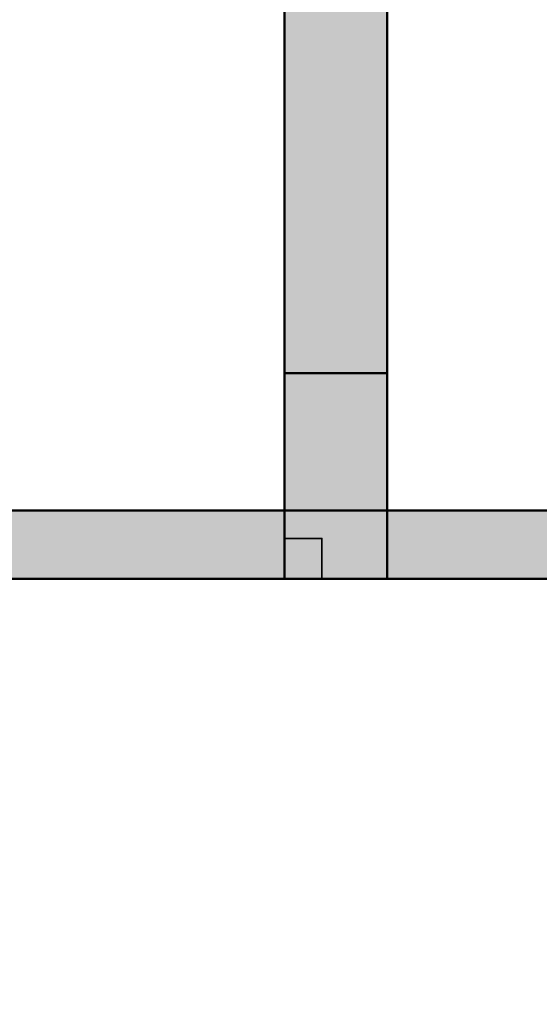
# Model space of a CAD drawing. Units: inches. Extents: x -7 to 1228, y -146 to 1091.
# Tile 64 of 88: x 611 to 656, y 531 to 617. Entities that reach past the tile are written whole.
import ezdxf

# ---------------------------------------------------------------- set-up
doc = ezdxf.new("R2010")
doc.units = ezdxf.units.IN
for name, color, linetype, lineweight in [('A-COLS', 6, 'Continuous', 35), ('A-WALL', 7, 'Continuous', 50), ('A-WALL-PATT', 251, 'Continuous', 13)]:
    doc.layers.add(name, color=color, linetype=linetype, lineweight=lineweight)

msp = doc.modelspace()

# ---------------------------------------------------------------- hatches: boundary and pattern name
at = {"layer": 'A-COLS'}
h = msp.add_hatch(color=256, dxfattribs=at)
h.dxf.hatch_style = 1
h.paths.add_polyline_path([(643, 586), (634, 586), (634, 571.546), (637.289, 571.546), (637.289, 568), (643, 568)])
h = msp.add_hatch(color=256, dxfattribs=at)
h.dxf.hatch_style = 1
h.paths.add_polyline_path([(637.289, 571.546), (634, 571.546), (634, 568), (637.289, 568)])
at = {"layer": 'A-WALL-PATT'}
h = msp.add_hatch(color=256, dxfattribs=at)
h.dxf.hatch_style = 1
h.paths.add_polyline_path([(69, 568), (60, 568), (60, 493), (63.289, 493), (69, 493)])
h.paths.add_polyline_path([(69, 662.405), (60, 662.405), (60, 586), (69, 586)], flags=17)
h.paths.add_polyline_path([(69, 723), (184, 723), (184, 734), (179, 734), (179, 728), (69, 728), (69, 741.623), (60, 741.623), (60, 698.405), (69, 698.405)], flags=17)
h.paths.add_polyline_path([(69, 782), (231, 782), (231, 728), (231, 723), (231, 586), (236, 586), (236, 787), (69, 787), (69, 800.126), (60, 800.126), (60, 765.623), (69, 765.623)])
h.paths.add_polyline_path([(184, 842), (189, 842), (189, 848), (173, 848), (173, 842), (179, 842), (179, 787), (184, 787)])
h.paths.add_polyline_path([(118.22, 69), (69, 69), (69, 60), (118.22, 60)])
h.paths.add_polyline_path([(227, 69), (154.22, 69), (154.22, 60), (227, 60)])
h.paths.add_polyline_path([(236, 60), (232.711, 60), (227, 60), (227, 36), (236, 36)])
h.paths.add_polyline_path([(389, 60), (380, 60), (380, 36), (389, 36)])
h.paths.add_polyline_path([(384, 181), (380, 181), (380, 115), (380, 78), (384, 78)])
h.paths.add_polyline_path([(380, 115), (334.547, 115), (334.547, 109), (380, 109)])
h.paths.add_polyline_path([(274.547, 115), (236, 115), (236, 201), (232.711, 201), (231, 201), (231, 78), (236, 78), (236, 109), (274.547, 109)])
h.paths.add_polyline_path([(69, 123), (60, 123), (60, 78), (69, 78)])
h.paths.add_polyline_path([(69, 201), (60, 201), (60, 159), (69, 159)])
h.paths.add_polyline_path([(143, 219), (69, 219), (69, 213), (143, 213)], flags=17)
h.paths.add_polyline_path([(189, 219), (184, 219), (184, 274), (231, 274), (231, 219), (236, 219), (236, 279), (184, 279), (184, 297), (179, 297), (179, 279), (69, 279), (69, 290.912), (60, 290.912), (60, 262.179), (69, 262.179), (69, 274), (179, 274), (179, 219), (173, 219), (173, 213), (189, 213)])
h.paths.add_polyline_path([(69, 238.179), (60, 238.179), (60, 219), (69, 219)], flags=17)
h.paths.add_polyline_path([(69, 333), (60, 333), (60, 314.912), (69, 314.912), (69, 316.965)])
h.paths.add_polyline_path([(190, 338), (184, 338), (69, 338), (69, 333), (179, 333), (179, 327), (184, 327), (184, 333.021), (190, 333.046)])
h.paths.add_polyline_path([(69, 386.806), (60, 386.806), (60, 351), (69, 351)])
h.paths.add_polyline_path([(69, 475), (60, 475), (60, 422.806), (69, 422.806)])
h.paths.add_polyline_path([(236, 475), (231, 475), (231, 351.238), (236, 351.238)])
h.paths.add_polyline_path([(384, 475), (380, 475), (380, 362), (384, 362)])
h.paths.add_polyline_path([(547, 307), (439, 307), (439, 356), (445, 356), (445, 362), (433, 362), (433, 307), (380, 307), (380, 244), (380, 241), (384, 241), (384, 301), (433, 301), (433, 277), (439, 277), (439, 301), (547, 301)])
h.paths.add_polyline_path([(547, 241), (439, 241), (439, 247), (433, 247), (433, 235), (547, 235)])
h.paths.add_polyline_path([(450, 69), (440.286, 69), (424.889, 69), (389, 69), (389, 60), (450, 60)])
h.paths.add_polyline_path([(547, 69), (486, 69), (486, 60), (547, 60)])
h.paths.add_polyline_path([(556, 148.268), (547, 148.268), (547, 78), (556, 78)])
h.paths.add_polyline_path([(556, 223), (547, 223), (547, 195), (547, 184.268), (556, 184.268)])
h.paths.add_polyline_path([(556, 311.192), (547, 311.192), (547, 273.075), (556, 273.075)])
h.paths.add_polyline_path([(556, 344), (552.711, 344), (547, 344), (547, 335.192), (556, 335.192)])
h.paths.add_polyline_path([(556, 249.075), (547, 249.075), (547, 241), (556, 241)])
h.paths.add_polyline_path([(547, 362), (475, 362), (475, 356), (547, 356)], flags=0)
h.paths.add_polyline_path([(556, 399.621), (547, 399.621), (547, 362), (556, 362)])
h.paths.add_polyline_path([(556, 475), (547, 475), (547, 435.621), (556, 435.621)])
h.paths.add_polyline_path([(547, 493), (389, 493), (389, 487), (547, 487)])
h.paths.add_polyline_path([(380, 493), (278, 493), (278, 487), (380, 487)])
h.paths.add_polyline_path([(227, 493), (69, 493), (69, 487), (227, 487)])
h.paths.add_polyline_path([(643, 122.445), (634, 122.445), (634, 78), (643, 78)])
h.paths.add_polyline_path([(702.5, 69), (692.786, 69), (677.389, 69), (643, 69), (643, 60), (702.5, 60)])
h.paths.add_polyline_path([(798, 69), (738.5, 69), (738.5, 60), (798, 60)])
h.paths.add_polyline_path([(807, 60), (803.711, 60), (798, 60), (798, 36), (807, 36)])
h.paths.add_polyline_path([(807, 109), (846.751, 109), (846.751, 115), (807, 115), (807, 159), (802, 159), (802, 78), (807, 78)])
h.paths.add_polyline_path([(807, 201), (802, 201), (802, 195), (807, 195)])
h.paths.add_polyline_path([(643, 201), (634, 201), (634, 158.445), (643, 158.445)])
h.paths.add_polyline_path([(756, 225), (751, 225), (751, 219), (643, 219), (643, 213), (756, 213)])
h.paths.add_polyline_path([(643, 240.848), (634, 240.848), (634, 219), (643, 219)])
h.paths.add_polyline_path([(643, 274), (643, 288.629), (634, 288.629), (634, 264.848), (643, 264.848)])
h.paths.add_polyline_path([(802, 279), (756, 279), (756, 297), (751, 297), (751, 279), (643, 279), (643, 274), (751, 274), (751, 255), (756, 255), (756, 274), (802, 274)])
h.paths.add_polyline_path([(807, 333), (803.711, 333), (802, 333), (802, 279), (802, 274), (802, 219), (807, 219)])
h.paths.add_polyline_path([(956, 182), (951, 182), (951, 115), (906.751, 115), (906.751, 109), (951, 109), (951, 78), (956, 78)])
h.paths.add_polyline_path([(960, 60), (951, 60), (951, 36), (960, 36)])
h.paths.add_polyline_path([(1021, 69), (1005.781, 69), (960, 69), (960, 60), (1021, 60)])
h.paths.add_polyline_path([(956, 224), (951, 224), (951, 218), (956, 218)])
h.paths.add_polyline_path([(956, 302), (1004, 302), (1004, 278), (1010, 278), (1010, 302), (1118, 302), (1118, 290.809), (1127, 290.809), (1127, 326.968), (1118, 326.968), (1118, 320.966), (1118, 307), (1010, 307), (1010, 356), (1016, 356), (1016, 362), (1004, 362), (1004, 307), (951, 307), (951, 244), (951, 242), (954.289, 242), (956, 242)])
h.paths.add_polyline_path([(643, 333), (634, 333), (634, 312.629), (643, 312.629), (643, 316.965)])
h.paths.add_polyline_path([(756, 338), (643, 338), (643, 333), (751, 333), (751, 327), (756, 327)])
h.paths.add_polyline_path([(643, 388), (634, 388), (634, 351), (643, 351)])
h.paths.add_polyline_path([(807, 357), (802, 357), (802, 351), (807, 351)])
h.paths.add_polyline_path([(807, 475), (802, 475), (802, 393), (807, 393)])
h.paths.add_polyline_path([(643, 475), (634, 475), (634, 424), (643, 424)])
h.paths.add_polyline_path([(798, 493), (643, 493), (643, 487), (798, 487)])
h.paths.add_polyline_path([(634, 493), (556, 493), (556, 487), (634, 487)])
h.paths.add_polyline_path([(813, 493), (807, 493), (807, 487), (813, 487)])
h.paths.add_polyline_path([(951, 493), (849, 493), (849, 487), (951, 487)])
h.paths.add_polyline_path([(956, 484), (951, 484), (951, 374), (956, 374)])
h.paths.add_polyline_path([(1109, 493), (969, 493), (969, 487), (1109, 487)])
h.paths.add_polyline_path([(1127, 484), (1118, 484), (1118, 450.641), (1127, 450.641)])
h.paths.add_polyline_path([(1127, 414.641), (1118, 414.641), (1118, 365), (1127, 365)])
h.paths.add_polyline_path([(1109, 362), (1046, 362), (1046, 356), (1109, 356)], flags=17)
h.paths.add_polyline_path([(1127, 356), (1123.454, 356), (1118, 356), (1118, 350.968), (1127, 350.968)], flags=0)
h.paths.add_polyline_path([(1127, 266.809), (1118, 266.809), (1118, 262.361), (1118, 242), (1127, 242)], flags=17)
h.paths.add_polyline_path([(1118, 242), (1010, 242), (1010, 248), (1004, 248), (1004, 237), (1118, 237)])
h.paths.add_polyline_path([(1127, 224), (1118, 224), (1118, 170), (1127, 170)])
h.paths.add_polyline_path([(1127, 134), (1118, 134), (1118, 78), (1127, 78)])
h.paths.add_polyline_path([(1118, 69), (1057, 69), (1057, 60), (1118, 60)])
h.paths.add_polyline_path([(227, 571.546), (227, 574), (69, 574), (69, 568), (227, 568)])
h.paths.add_polyline_path([(380, 571.546), (380, 574), (278, 574), (278, 568), (380, 568)])
h.paths.add_polyline_path([(242, 574), (236, 574), (236, 568), (242, 568)])
h.paths.add_polyline_path([(547, 571.546), (547, 574), (389, 574), (389, 568), (547, 568)])
h.paths.add_polyline_path([(384, 733), (380, 733), (380, 586), (384, 586)])
h.paths.add_polyline_path([(556, 646), (634, 646), (634, 655), (547, 655), (547, 586), (556, 586)])
h.paths.add_polyline_path([(634, 574), (556, 574), (556, 568), (634, 568)])
h.paths.add_polyline_path([(643, 655), (634, 655), (634, 586), (643, 586)])
h.paths.add_polyline_path([(798, 574), (643, 574), (643, 568), (798, 568)])
h.paths.add_polyline_path([(643, 663.854), (634, 663.854), (634, 655), (643, 655)])
h.paths.add_polyline_path([(556, 676.967), (547, 676.967), (547, 655), (556, 655)])
h.paths.add_polyline_path([(556, 733), (547, 733), (547, 712.967), (556, 712.967)])
h.paths.add_polyline_path([(643, 710), (634, 710), (634, 699.854), (643, 699.854)])
h.paths.add_polyline_path([(807, 668), (802, 668), (802, 586), (807, 586)])
h.paths.add_polyline_path([(951, 574), (849, 574), (849, 568), (951, 568)])
h.paths.add_polyline_path([(956, 691), (951, 691), (951, 577), (956, 577)])
h.paths.add_polyline_path([(1109, 574), (969, 574), (969, 568), (1109, 568)])
h.paths.add_polyline_path([(1127, 643.403), (1118, 643.403), (1118, 577), (1127, 577)])
h.paths.add_polyline_path([(1127, 568), (1123.454, 568), (1118, 568), (1118, 493), (1127, 493)])
h.paths.add_polyline_path([(1127, 733), (1118, 733), (1118, 679.403), (1127, 679.403)])
h.paths.add_polyline_path([(1127, 777.348), (1118, 777.348), (1118, 770.035), (1118, 751), (1127, 751)], flags=17)
h.paths.add_polyline_path([(1118, 751), (1010, 751), (1010, 757), (1004, 757), (1004, 745), (1118, 745)])
h.paths.add_polyline_path([(956, 811), (1004, 811), (1004, 787), (1010, 787), (1010, 811), (1017.874, 811), (1017.874, 811.627, -0.414214), (1018.247, 812), (1031.978, 812, -0.414214), (1032.351, 811.627), (1032.351, 811), (1118, 811), (1118, 801.348), (1127, 801.348), (1127, 834.685), (1118, 834.685), (1118, 830.238), (1118, 817), (1010, 817), (1010, 866), (1016, 866), (1016, 872), (1004, 872), (1004, 817), (956, 817), (956, 866), (951, 866), (951, 751), (954.289, 751), (956, 751)])
h.paths.add_polyline_path([(1118, 872), (1046, 872), (1046, 866), (1118, 866)], flags=17)
h.paths.add_polyline_path([(1127, 924.711), (1118, 924.711), (1118, 884), (1127, 884)])
h.paths.add_polyline_path([(1127, 866), (1123.711, 866), (1118, 866), (1118, 858.685), (1127, 858.685)], flags=17)
h.paths.add_polyline_path([(956, 983), (951, 983), (951, 952), (807, 952), (807, 983), (802, 983), (802, 902), (807, 902), (807, 946), (951, 946), (951, 884), (956, 884)])
h.paths.add_polyline_path([(807, 842), (802, 842), (802, 787), (756, 787), (756, 806), (751, 806), (751, 787), (643, 787), (643, 782), (751, 782), (751, 764), (756, 764), (756, 782), (802, 782), (802, 728), (807, 728)])
h.paths.add_polyline_path([(756, 848), (643, 848), (643, 842), (751, 842), (751, 836), (756, 836)])
h.paths.add_polyline_path([(756, 734), (751, 734), (751, 728), (643, 728), (643, 723), (756, 723)])
h.paths.add_polyline_path([(643, 749.791), (634, 749.791), (634, 728), (637.289, 728), (643, 728)])
h.paths.add_polyline_path([(643, 805.405), (634, 805.405), (634, 773.791), (643, 773.791)])
h.paths.add_polyline_path([(643, 896.663), (634, 896.663), (634, 860), (637.289, 860), (643, 860)])
h.paths.add_polyline_path([(643, 842), (634, 842), (634, 829.405), (643, 829.405)])
h.paths.add_polyline_path([(643, 983), (634, 983), (634, 932.663), (643, 932.663)])
h.paths.add_polyline_path([(1127, 983), (1118, 983), (1118, 960.711), (1127, 960.711)])
h.paths.add_polyline_path([(1118, 1001), (1077.525, 1001), (1077.525, 992), (1118, 992)])
h.paths.add_polyline_path([(1041.525, 1001), (960, 1001), (960, 992), (1041.525, 992)])
h.paths.add_polyline_path([(960, 1025), (951, 1025), (951, 1001), (954.289, 1001), (960, 1001)])
h.paths.add_polyline_path([(807, 1025), (798, 1025), (798, 1001), (807, 1001)])
h.paths.add_polyline_path([(798, 1001), (738.5, 1001), (738.5, 992), (798, 992)])
h.paths.add_polyline_path([(702.5, 1001), (643, 1001), (643, 992), (702.5, 992)])
h.paths.add_polyline_path([(547, 1001), (499.113, 1001), (499.113, 992), (547, 992)])
h.paths.add_polyline_path([(463.113, 1001), (389, 1001), (389, 992), (463.113, 992)])
h.paths.add_polyline_path([(389, 1025), (380, 1025), (380, 1022), (380, 1001), (383.289, 1001), (389, 1001)])
h.paths.add_polyline_path([(236, 1025), (227, 1025), (227, 1001), (236, 1001)])
h.paths.add_polyline_path([(236, 983), (231, 983), (231, 860), (236, 860)])
h.paths.add_polyline_path([(274.547, 952), (236, 952), (236, 946), (274.547, 946)])
h.paths.add_polyline_path([(380, 952), (334.547, 952), (334.547, 946), (380, 946)])
h.paths.add_polyline_path([(384, 983), (380, 983), (380, 884), (383.289, 884), (384, 884)])
h.paths.add_polyline_path([(227, 1001), (155.012, 1001), (155.012, 992), (162.875, 992), (227, 992)])
h.paths.add_polyline_path([(119.012, 1001), (69, 1001), (69, 992), (119.012, 992)])
h.paths.add_polyline_path([(69, 983), (60, 983), (60, 922.987), (69, 922.987)])
h.paths.add_polyline_path([(69, 886.987), (60, 886.987), (60, 860), (63.289, 860), (69, 860)])
h.paths.add_polyline_path([(143, 848), (69, 848), (69, 842), (143, 842)])

# ---------------------------------------------------------------- linework, layer by layer
at = {"layer": 'A-COLS'}
msp.add_lwpolyline([(634, 568), (637.289, 568), (637.289, 571.546), (634, 571.546)], close=True, dxfattribs=at)
at = {"layer": 'A-WALL'}
for p, q in [((634, 568), (634, 1001)), ((643, 568), (643, 1001)), ((643, 723), (643, 568)), ((634, 646), (634, 568)), ((643, 586), (634, 586)), ((634, 586), (634, 574)), ((643, 568), (643, 586)), ((813, 574), (556, 574)), ((634, 571.546), (634, 568)), ((813, 568), (556, 568)), ((634, 568), (643, 568))]:
    msp.add_line(p, q, dxfattribs=at)

doc.saveas('drawing.dxf')
